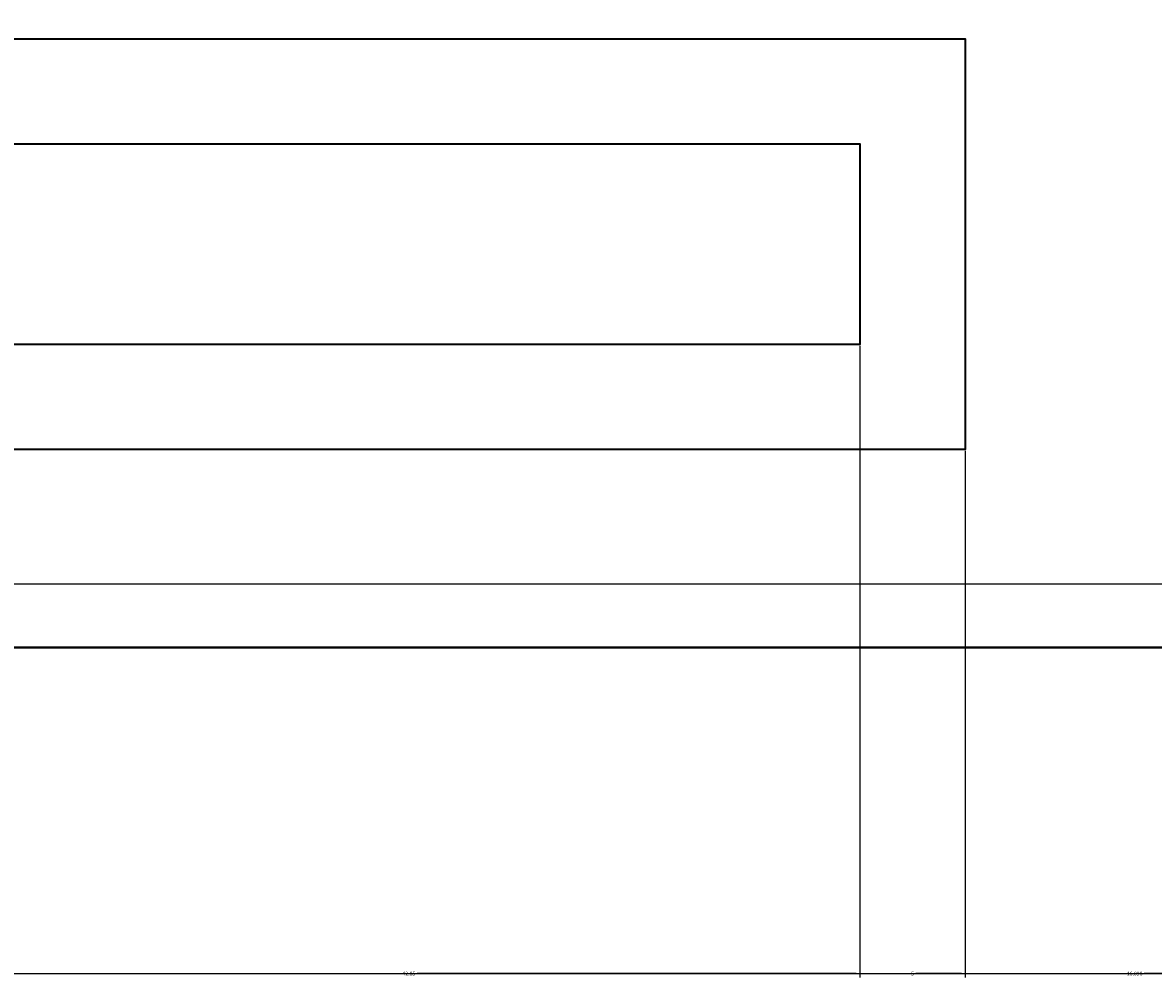
# Model space of a CAD drawing. Units: inches. Extents: x -6 to 289, y -8 to 323.
# Tile 8 of 107: x 48 to 102, y -8 to 37. Entities that reach past the tile are written whole.
import ezdxf

# ---------------------------------------------------------------- set-up
doc = ezdxf.new("R2010")
doc.units = ezdxf.units.IN
doc.header["$MEASUREMENT"] = 0
doc.layers.add('A-ANNO-DIMS', color=2, linetype='Continuous', lineweight=18)
doc.layers.add('A-ELEV', color=7, linetype='Continuous', lineweight=35)
doc.styles.get("Standard").update_dxf_attribs({"font": 'arial.ttf'})
doc.dimstyles.get("Standard").update_dxf_attribs({"dimtxt": 0.18, "dimasz": 0.18, "dimexe": 0.18, "dimexo": 0.0625, "dimgap": 0.09, "dimtad": 0, "dimtih": 1, "dimtoh": 1, "dimdec": 4, "dimzin": 0, "dimdsep": 46, "dimtxsty": 'Standard', "dimcen": 0.09, "dimadec": 0, "dimazin": 0, "dimtfac": 1, "dimtdec": 4, "dimtofl": 0, "dimtmove": 0, "dimatfit": 3, "dimfxl": 1, "dimtolj": 1, "dimtzin": 0, "dimarcsym": 0})

# ---------------------------------------------------------------- blocks, each defined once
blk = doc.blocks.new('*D16')
at = {"layer": 'A-ANNO-DIMS', "color": 0, "lineweight": -2, "transparency": 16777216}
for p, q in [((9.943, 68.37), (9.943, -8.391)), ((272.973, 68.37), (272.973, -8.391)), ((10.123, -8.211), (140.993, -8.211)), ((272.793, -8.211), (141.923, -8.211))]:
    blk.add_line(p, q, dxfattribs=at)
at = {"layer": 'A-ANNO-DIMS', "color": 0, "transparency": 16777216}
for points in [[(10.123, -8.181), (10.123, -8.241), (9.943, -8.211)], [(272.793, -8.181), (272.793, -8.241), (272.973, -8.211)]]:
    blk.add_solid(points, dxfattribs=at)
at = {"layer": 'Defpoints', "color": 0, "transparency": 16777216}
for p in [(9.943, 68.432), (272.973, 68.432), (272.973, -8.211)]:
    blk.add_point(p, dxfattribs=at)
at = {"layer": 'A-ANNO-DIMS', "color": 0, "transparency": 16777216, "insert": (141.458, -8.211), "char_height": 0.18, "attachment_point": 5}
blk.add_mtext('\\A1;263.03', dxfattribs=at)
blk = doc.blocks.new('*D53')
at = {"layer": 'A-ANNO-DIMS', "color": 0, "lineweight": -2, "transparency": 16777216}
for p, q in [((44.709, 21.629), (44.709, -8.391)), ((87.562, 21.629), (87.562, -8.391)), ((44.889, -8.211), (65.738, -8.211)), ((87.382, -8.211), (66.534, -8.211))]:
    blk.add_line(p, q, dxfattribs=at)
at = {"layer": 'A-ANNO-DIMS', "color": 0, "transparency": 16777216}
for points in [[(44.889, -8.181), (44.889, -8.241), (44.709, -8.211)], [(87.382, -8.181), (87.382, -8.241), (87.562, -8.211)]]:
    blk.add_solid(points, dxfattribs=at)
at = {"layer": 'Defpoints', "color": 0, "transparency": 16777216}
for p in [(44.709, 21.692), (87.562, 21.692), (87.562, -8.211)]:
    blk.add_point(p, dxfattribs=at)
at = {"layer": 'A-ANNO-DIMS', "color": 0, "transparency": 16777216, "insert": (66.136, -8.211), "char_height": 0.18, "attachment_point": 5}
blk.add_mtext('\\A1;42.85', dxfattribs=at)
blk = doc.blocks.new('*D54')
at = {"layer": 'A-ANNO-DIMS', "color": 0, "lineweight": -2, "transparency": 16777216}
for p, q in [((87.562, 21.629), (87.562, -8.391)), ((92.562, 16.629), (92.562, -8.391)), ((87.742, -8.211), (89.913, -8.211)), ((92.382, -8.211), (90.212, -8.211))]:
    blk.add_line(p, q, dxfattribs=at)
at = {"layer": 'A-ANNO-DIMS', "color": 0, "transparency": 16777216}
for points in [[(87.742, -8.181), (87.742, -8.241), (87.562, -8.211)], [(92.382, -8.181), (92.382, -8.241), (92.562, -8.211)]]:
    blk.add_solid(points, dxfattribs=at)
at = {"layer": 'Defpoints', "color": 0, "transparency": 16777216}
for p in [(87.562, 21.692), (92.562, 16.692), (92.562, -8.211)]:
    blk.add_point(p, dxfattribs=at)
at = {"layer": 'A-ANNO-DIMS', "color": 0, "transparency": 16777216, "insert": (90.062, -8.211), "char_height": 0.18, "attachment_point": 5}
blk.add_mtext('\\A1;5', dxfattribs=at)
blk = doc.blocks.new('*D55')
at = {"layer": 'A-ANNO-DIMS', "color": 0, "lineweight": -2, "transparency": 16777216}
for p, q in [((92.562, 16.629), (92.562, -8.391)), ((108.66, 7.226), (108.66, -8.391)), ((92.742, -8.211), (100.156, -8.211)), ((108.48, -8.211), (101.067, -8.211))]:
    blk.add_line(p, q, dxfattribs=at)
at = {"layer": 'A-ANNO-DIMS', "color": 0, "transparency": 16777216}
for points in [[(92.742, -8.181), (92.742, -8.241), (92.562, -8.211)], [(108.48, -8.181), (108.48, -8.241), (108.66, -8.211)]]:
    blk.add_solid(points, dxfattribs=at)
at = {"layer": 'Defpoints', "color": 0, "transparency": 16777216}
for p in [(92.562, 16.692), (108.66, 7.289), (108.66, -8.211)]:
    blk.add_point(p, dxfattribs=at)
at = {"layer": 'A-ANNO-DIMS', "color": 0, "transparency": 16777216, "insert": (100.611, -8.211), "char_height": 0.18, "attachment_point": 5}
blk.add_mtext('\\A1;16.098', dxfattribs=at)
blk = doc.blocks.new('*D83')
at = {"layer": 'A-ANNO-DIMS', "color": 0, "lineweight": -2, "transparency": 16777216}
for p, q in [((123.945, 10.289), (-5.737, 10.289)), ((-5.557, 10.109), (-5.557, 8.971)), ((-5.557, 7.469), (-5.557, 8.607)), ((120.945, 7.289), (-5.737, 7.289))]:
    blk.add_line(p, q, dxfattribs=at)
at = {"layer": 'A-ANNO-DIMS', "color": 0, "transparency": 16777216}
for points in [[(-5.587, 10.109), (-5.527, 10.109), (-5.557, 10.289)], [(-5.587, 7.469), (-5.527, 7.469), (-5.557, 7.289)]]:
    blk.add_solid(points, dxfattribs=at)
at = {"layer": 'Defpoints', "color": 0, "transparency": 16777216}
for p in [(-5.557, 10.289), (124.008, 10.289), (121.008, 7.289)]:
    blk.add_point(p, dxfattribs=at)
at = {"layer": 'A-ANNO-DIMS', "color": 0, "transparency": 16777216, "insert": (-5.557, 8.789), "char_height": 0.18, "attachment_point": 5}
blk.add_mtext('\\A1;3', dxfattribs=at)
blk = doc.blocks.new('*D84')
at = {"layer": 'A-ANNO-DIMS', "color": 0, "lineweight": -2, "transparency": 16777216}
for p, q in [((123.945, 48.085), (-5.737, 48.085)), ((-5.557, 47.905), (-5.557, 29.369)), ((-5.557, 10.469), (-5.557, 29.005)), ((123.945, 10.289), (-5.737, 10.289))]:
    blk.add_line(p, q, dxfattribs=at)
at = {"layer": 'A-ANNO-DIMS', "color": 0, "transparency": 16777216}
for points in [[(-5.587, 47.905), (-5.527, 47.905), (-5.557, 48.085)], [(-5.587, 10.469), (-5.527, 10.469), (-5.557, 10.289)]]:
    blk.add_solid(points, dxfattribs=at)
at = {"layer": 'Defpoints', "color": 0, "transparency": 16777216}
for p in [(-5.557, 48.085), (124.008, 48.085), (124.008, 10.289)]:
    blk.add_point(p, dxfattribs=at)
at = {"layer": 'A-ANNO-DIMS', "color": 0, "transparency": 16777216, "insert": (-5.557, 29.187), "char_height": 0.18, "attachment_point": 5}
blk.add_mtext('\\A1;37.8', dxfattribs=at)

msp = doc.modelspace()

# ---------------------------------------------------------------- linework, layer by layer
at = {"layer": 'A-ELEV'}
msp.add_line((19.1638, 7.2888), (271.1638, 7.2888), dxfattribs=at)
for points in [[(24.317, 49.3604), (108.6602, 49.3604), (108.6602, 7.2888), (24.317, 7.2888)], [(39.709, 36.2133), (92.5623, 36.2133), (92.5623, 16.6917), (39.709, 16.6917)], [(44.709, 31.2133), (87.5623, 31.2133), (87.5623, 21.6917), (44.709, 21.6917)]]:
    msp.add_lwpolyline(points, close=True, dxfattribs=at)

# ---------------------------------------------------------------- dimensions: what is measured, and where the dimension line sits
at = {"layer": 'A-ANNO-DIMS'}
for base, p1, p2, override, picture, middle in [((272.9733, -8.2112), (9.943, 68.4322), (272.9733, 68.4322), {"dimdec": 2, "dimlfac": 1, "dimrnd": 0, "dimzin": 0, "dimdsep": 46, "dimlunit": 2}, '*D16', (141.4581, -8.2112)), ((87.5623, -8.2112), (44.709, 21.6917), (87.5623, 21.6917), {"dimdec": 2, "dimlfac": 1, "dimrnd": 0, "dimzin": 0, "dimdsep": 46, "dimlunit": 2}, '*D53', (66.1357, -8.2112)), ((92.5623, -8.2112), (87.5623, 21.6917), (92.5623, 16.6917), {"dimdec": 0, "dimlfac": 1, "dimrnd": 0, "dimzin": 0, "dimdsep": 46, "dimlunit": 2}, '*D54', (90.0623, -8.2112)), ((108.6602, -8.2112), (92.5623, 16.6917), (108.6602, 7.2888), {"dimdec": 3, "dimlfac": 1, "dimrnd": 0, "dimzin": 0, "dimdsep": 46, "dimlunit": 2}, '*D55', (100.6113, -8.2112))]:
    dim = msp.add_linear_dim(base=base, p1=p1, p2=p2, dimstyle='Standard', override=override, dxfattribs=at)
    dim.commit()
    dim.dimension.update_dxf_attribs({"geometry": picture, "text_midpoint": middle})
for base, p1, p2, override, picture, middle in [((-5.557, 48.0851), (124.008, 10.2888), (124.008, 48.0851), {"dimdec": 1, "dimlfac": 1, "dimrnd": 0, "dimzin": 0, "dimdsep": 46, "dimlunit": 2}, '*D84', (-5.557, 29.187)), ((-5.557, 10.2888), (121.008, 7.2888), (124.008, 10.2888), {"dimdec": 0, "dimlfac": 1, "dimrnd": 0, "dimzin": 0, "dimdsep": 46, "dimlunit": 2}, '*D83', (-5.557, 8.7888))]:
    dim = msp.add_linear_dim(base=base, p1=p1, p2=p2, angle=90, dimstyle='Standard', override=override, dxfattribs=at)
    dim.commit()
    dim.dimension.update_dxf_attribs({"geometry": picture, "text_midpoint": middle})

doc.saveas('drawing.dxf')
